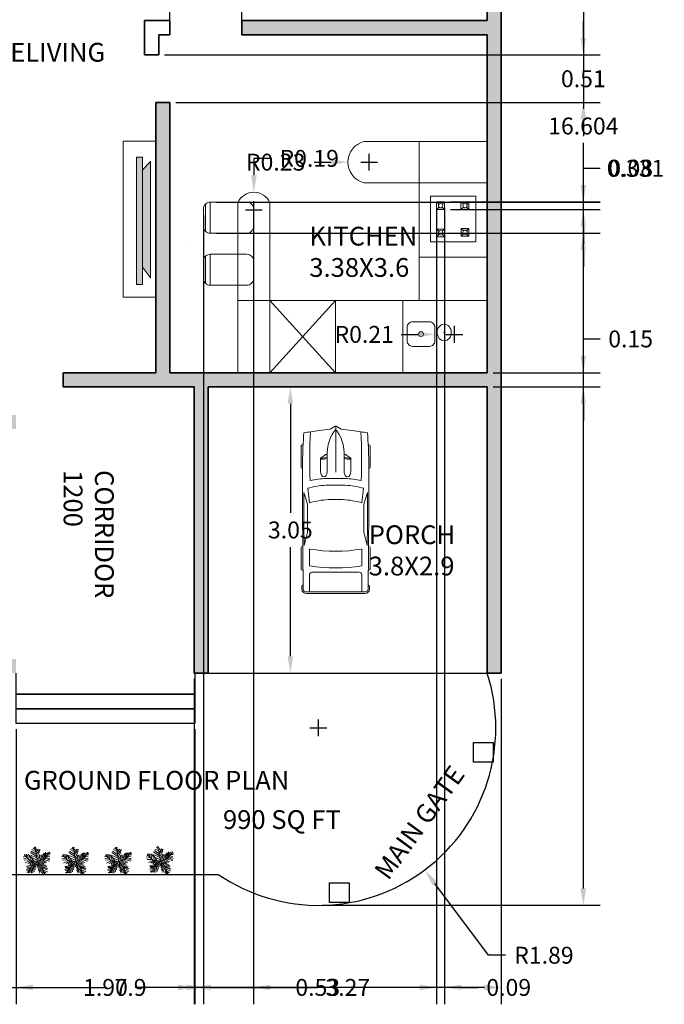
# Model space of a CAD drawing. Units: metres. Extents: x 36 to 56493, y 9 to 42849.
# Tile 2 of 5: x 56486.02 to 56492.89, y 42829.4 to 42839.88. Entities that reach past the tile are written whole.
import ezdxf

# ---------------------------------------------------------------- set-up
doc = ezdxf.new("R2010")
doc.units = ezdxf.units.M
doc.header["$MEASUREMENT"] = 0
for name, color, linetype, lineweight in [('A-ANNO-DIMS', 2, 'Continuous', 18), ('A-ANNO-TEXT', 7, 'Continuous', 25), ('A-AREA-IDEN', 7, 'Continuous', 18), ('A-EQPM', 8, 'Continuous', 18), ('A-EQPM-PATT', 8, 'Continuous', 13), ('A-FLOR', 7, 'Continuous', 25), ('A-FLOR-CASE', 9, 'Continuous', 18), ('A-FLOR-FIXT', 8, 'Continuous', 18), ('A-FLOR-STRS', 2, 'Continuous', 25), ('A-FURN', 8, 'Continuous', 18), ('A-WALL', 7, 'Continuous', 35), ('C-PKNG-VEHC', 9, 'Continuous', 13), ('C-PROP', 7, 'Continuous', 25), ('L-PLNT', 3, 'Continuous', 13)]:
    doc.layers.add(name, color=color, linetype=linetype, lineweight=lineweight)
doc.layers.add('A-WALL-PATT', color=30, linetype='Continuous', lineweight=13, true_color=0xf26722)
doc.styles.get("Standard").update_dxf_attribs({"font": 'arial.ttf'})
doc.dimstyles.get("Standard").update_dxf_attribs({"dimtxt": 0.18, "dimasz": 0.18, "dimexe": 0.18, "dimexo": 0.0625, "dimgap": 0.09, "dimtad": 0, "dimtih": 1, "dimtoh": 1, "dimdec": 0, "dimzin": 0, "dimdsep": 46, "dimtxsty": 'Standard', "dimcen": 0.09, "dimadec": 0, "dimazin": 0, "dimtfac": 1, "dimtdec": 0, "dimtofl": 0, "dimtmove": 0, "dimatfit": 3, "dimfxl": 1, "dimtolj": 1, "dimtzin": 0, "dimarcsym": 0})

# ---------------------------------------------------------------- blocks, each defined once
blk = doc.blocks.new('*U4')
for p, q in [((-5.114, 28.097), (-24.676, 40.636)), ((-7.288, 39.707), (-21.778, 46.673)), ((-8.737, 47.138), (-17.069, 52.711)), ((-10.186, 53.64), (-13.084, 55.962)), ((0, 0), (-10.5, 57)), ((-9.099, 51.782), (-6.563, 55.962)), ((-7.65, 43.423), (-2.578, 49.46)), ((-5.839, 35.992), (4.667, 48.067)), ((-5.114, 27.632), (10.463, 46.673)), ((-47.498, 19.737), (-55.83, 18.344)), ((-40.615, 13.7), (-55.105, 10.913)), ((-31.5, 4.5), (-52.5, 25.5)), ((-33.37, 6.269), (-52.207, 5.34)), ((-48.585, 21.131), (-49.309, 29.026)), ((-28.299, 3.483), (-47.86, -5.805)), ((-43.513, 28.561), (-42.427, 15.558)), ((-38.442, 26.239), (-34.819, 7.663)), ((-21.416, 3.018), (-38.079, -8.128)), ((-35.544, 28.097), (-24.314, 3.947)), ((0, 0), (-31.5, 4.5)), ((-14.533, 2.09), (-30.834, 25.31)), ((-15.982, 2.09), (-30.11, -9.521)), ((-3.665, 19.273), (-27.574, 35.527)), ((-24.314, 23.917), (-2.941, 13.7)), ((0, 0), (-22.5, -19.5)), ((-6.563, 1.161), (-21.416, -8.128)), ((-20.691, 13.7), (-1.129, 4.876)), ((-2.941, 16.486), (8.652, 37.85)), ((-1.129, 6.734), (9.014, 26.704)), ((0, 0), (27, 9)), ((0, 0), (18, -22.5)), ((3.942, 1.625), (11.187, 24.381)), ((6.478, 1.625), (26.04, -8.592)), ((10.101, 3.483), (17.708, 26.239)), ((11.187, 3.483), (30.749, -5.805)), ((16.259, 5.805), (23.142, 31.348)), ((18.07, 5.805), (35.096, -3.483)), ((22.055, 7.198), (27.489, 32.277)), ((24.229, 7.663), (46.688, 1.625)), ((27, 9), (48, 36)), ((27.127, 9.056), (31.112, 35.992)), ((29.662, 12.307), (48.137, 6.269)), ((31.836, 30.883), (32.561, 16.486)), ((33.285, 16.486), (48.862, 10.913)), ((35.096, 32.741), (37.27, 22.524)), ((36.183, 19.737), (48.137, 17.88)), ((38.719, 34.134), (41.979, 28.561)), ((40.53, 25.775), (48.862, 24.846)), ((43.791, 29.954), (51.036, 30.883)), ((44.153, 36.456), (45.239, 32.741)), ((-17.431, -15.094), (-42.789, -18.809)), ((-28.299, -29.026), (-42.789, -31.348)), ((-24.314, -21.596), (-42.427, -22.06)), ((-30.834, -34.135), (-42.427, -35.528)), ((-26.849, -26.24), (-40.253, -25.775)), ((-22.5, -19.5), (-37.5, -45)), ((-32.646, -36.921), (-31.921, -44.352)), ((-15.257, -12.772), (-30.11, -12.772)), ((-29.023, -30.884), (-27.936, -43.887)), ((-25.038, -23.918), (-22.865, -45.281)), ((-20.691, -18.345), (-17.793, -44.352)), ((-6.563, -5.805), (-19.967, -9.985)), ((-17.069, -15.094), (-12.721, -40.172)), ((-13.446, -11.378), (-8.737, -32.741)), ((-9.461, -8.592), (-6.201, -23.453)), ((-4.752, -3.483), (-3.665, -14.629)), ((2.493, -3.019), (-1.491, -20.202)), ((1.769, -2.555), (24.229, -9.521)), ((5.029, -6.27), (2.131, -25.775)), ((9.014, -11.378), (3.58, -35.992)), ((14.085, -16.951), (6.478, -40.172)), ((7.565, -9.056), (32.198, -14.629)), ((18.07, -22.524), (8.289, -45.745)), ((12.274, -15.094), (36.907, -18.809)), ((20.244, -30.419), (15.897, -44.816)), ((16.259, -19.738), (36.183, -22.989)), ((18, -22.5), (27, -52.5)), ((18.433, -22.524), (40.53, -29.026)), ((19.157, -25.311), (38.719, -33.206)), ((22.78, -37.85), (19.519, -48.532)), ((21.331, -32.741), (39.081, -40.636)), ((22.78, -38.314), (34.372, -44.816)), ((-34.457, -39.708), (-40.978, -42.494)), ((24.591, -45.745), (23.142, -50.854)), ((24.591, -43.423), (30.749, -47.603)), ((26.764, -49.925), (28.213, -50.854))]:
    blk.add_line(p, q)
blk = doc.blocks.new('*U6')
for p, q in [((21.1, 37.4), (21.1, 36.8)), ((46.6, 38.9), (22.4, 38.9)), ((47.8, 37.4), (47.8, 37.4)), ((88, 31.9), (74.8, 35.9)), ((134.3, 35.6), (119.3, 31.8)), ((135.5, 37.1), (135.5, 37.4)), ((136.7, 38.9), (160.9, 38.9)), ((162.1, 37.4), (162.1, 36.8)), ((186.5, -33.5), (186.5, 33.5)), ((70, 31.5), (86.4, 29.4)), ((138.4, 29.4), (157.2, 29.4)), ((164.5, 26.4), (164.5, -26.4)), ((186.5, 29.4), (167, 29.4)), ((188.4, -32.8), (188.4, 32.8)), ((32.1, 9.5), (32.1, 11.2)), ((32.3, 11.6), (36.1, 17.2)), ((36.1, 17.2), (50.9, 17.2)), ((3.3, 6.1), (0.1, 0.4)), ((29.8, 9.5), (51.7, 9.5)), ((58.9, -10.8), (58.9, 10.8)), ((66.6, -10.5), (66.6, 10.5)), ((82.7, 8.5), (82.7, -8.5)), ((186.5, -10.5), (186.5, 10.5)), ((0, 0), (51.7, 0)), ((0.1, -0.4), (3.3, -6.1)), ((29.8, -9.5), (51.7, -9.5)), ((32.1, -9.5), (32.1, -11.2)), ((32.3, -11.6), (36.1, -17.2)), ((36.1, -17.2), (50.9, -17.2)), ((86.4, -29.4), (70, -31.5)), ((88, -31.9), (74.8, -35.9)), ((134.3, -35.6), (119.3, -31.8)), ((157.2, -29.4), (138.4, -29.4)), ((167, -29.4), (186.5, -29.4)), ((21.1, -37.4), (21.1, -36.8)), ((46.6, -38.9), (22.4, -38.9)), ((47.8, -37.4), (47.8, -37.4)), ((135.5, -37.1), (135.5, -37.4)), ((136.7, -38.9), (160.9, -38.9)), ((162.1, -37.4), (162.1, -36.8))]:
    blk.add_line(p, q)
for centre, major_axis, ratio, start_param, end_param in [((266, -27.5), (0, 313.3), 0.842304, 1.367076, 1.39176), ((41.2, -490.9), (0, 528.2), 0.842304, 0.00281, 0.075598), ((22.4, 37.4), (0, -1.48), 0.842304, 3.141593, 4.712389), ((64.5, -10555.6), (0, 10593), 0.842304, -0.013397, 0.002797), ((46.6, 37.4), (0, 1.48), 0.842304, -1.570796, 0), ((64.5, -10555.6), (0, -10591.5), 0.842304, 3.133765, 3.140441), ((136.7, 37.4), (0, -1.48), 0.842304, 3.141593, 4.712389), ((160.9, 37.4), (0, 1.48), 0.842304, -1.570796, 0), ((180.6, 35.8), (0, 2.22), 0.842304, -0.013017, 1.249894), ((64.5, -10556.4), (0, 10595.3), 0.842304, -0.013397, -0.013017), ((184, 32.8), (0, -5.25), 0.842304, 1.570796, 3.128196), ((184, 33.5), (0, -2.96), 0.842304, 1.570796, 3.128196), ((259.2, -27.5), (0, -305.3), 0.842304, 4.528606, 4.561838), ((37.5, -594), (0, -623.3), 0.842304, 3.096046, 3.200911), ((134.4, 5.4), (0, -89.8), 0.842304, 4.449482, 4.652344), ((135.3, 5.4), (0, 81.8), 0.842304, 1.245306, 1.50788), ((149.6, 2.8), (0, -79.6), 0.842304, 4.372215, 4.640744), ((95.8, -3666.4), (0, -3698.2), 0.842304, 3.134049, 3.144098), ((17.1, 0), (0, 147), 0.842304, 4.511394, 4.913384), ((35.9, 0), (0, 147), 0.842304, 4.511394, 4.913384), ((167, 26.4), (0, 2.96), 0.842304, 0, 1.570796), ((-204.5, 52.4), (0, -251), 0.842304, 1.385369, 1.434372), ((32.7, 11.2), (0, 0.74), 0.842304, 0.879714, 1.570796), ((13, 17), (0, 27.4), 0.842304, 4.435146, 4.718221), ((14.2, 17), (0, 27.4), 0.842304, 4.435146, 4.718221), ((50.8, 13.3), (6.34, -0.36), 0.603834, -1.395552, 1.581315), ((0.6, 0), (0, -0.74), 0.842304, 4.131459, 5.293319), ((29.8, -46.7), (0, 56.2), 0.842304, 0, 0.590319), ((-204.5, -52.4), (0, 251), 0.842304, -1.434372, -1.385369), ((29.8, 46.7), (0, 56.2), 0.842304, 2.551274, 3.141593), ((13, -17), (0, -27.4), 0.842304, 1.564964, 1.848039), ((14.2, -17), (0, -27.4), 0.842304, 1.564964, 1.848039), ((134.4, -5.4), (0, -89.8), 0.842304, -1.510751, -1.307889), ((135.3, -5.4), (0, -81.8), 0.842304, -1.50788, -1.245306), ((149.6, -2.8), (0, -79.6), 0.842304, -1.499151, -1.230623), ((259.2, 27.5), (0, 305.3), 0.842304, 1.721348, 1.754579), ((32.7, -11.2), (0, -0.74), 0.842304, 4.712389, 5.403472), ((266, 27.5), (0, 313.3), 0.842304, 1.749832, 1.774517), ((37.5, 594), (0, -623.3), 0.842304, -0.059319, 0.045547), ((95.8, 3666.4), (0, -3698.2), 0.842304, -0.002505, 0.007544), ((167, -26.4), (0, -2.96), 0.842304, 4.712389, 6.283185), ((184, -32.8), (0, -5.25), 0.842304, 0.013397, 1.570796), ((41.2, 490.9), (0, -528.2), 0.842304, -0.075598, -0.00281), ((22.4, -37.4), (0, 1.48), 0.842304, 1.570796, 3.141593), ((64.5, 10555.6), (0, 10593), 0.842304, 3.138796, 3.15499), ((46.6, -37.4), (0, -1.48), 0.842304, 0, 1.570796), ((64.5, 10555.6), (0, -10591.5), 0.842304, 0.001152, 0.007828), ((136.7, -37.4), (0, -1.48), 0.842304, -1.570796, 0), ((160.9, -37.4), (0, 1.48), 0.842304, 3.141593, 4.712389), ((180.6, -35.8), (0, -2.22), 0.842304, -1.249894, 0.013017), ((64.5, 10556.4), (0, 10595.3), 0.842304, 3.15461, 3.15499), ((184, -33.5), (0, 2.96), 0.842304, 3.15499, 4.712389)]:
    blk.add_ellipse(centre, major_axis=major_axis, ratio=ratio, start_param=start_param, end_param=end_param)
at = {"extrusion": (0, 0, -1)}
blk.add_ellipse((50.8, -13.3), major_axis=(6.34, 0.36), ratio=0.603834, start_param=-1.395552, end_param=1.581315, dxfattribs=at)
blk = doc.blocks.new('HOB-BURNER')
for p, q in [((0, 0.081), (0.026, 0.057)), ((0, 0), (0.026, 0.025)), ((0.026, 0.025), (0.026, 0.025)), ((0.085, 0.081), (0.059, 0.057)), ((0.085, 0), (0.059, 0.025))]:
    blk.add_line(p, q)
blk.add_lwpolyline([(0, 0.081), (0, 0.081), (0.085, 0.081), (0.085, 0.081), (0.085, 0), (0.085, 0), (0, 0), (0, 0)], close=True)
blk.add_circle((0.043, 0.041), 0.0232)
blk = doc.blocks.new('COUNTER-STOOL')
for p, q in [((0.073, 0.331), (0.073, 0)), ((0.022, 0.31), (0.022, 0.022))]:
    blk.add_line(p, q)
blk.add_lwpolyline([(0, 0.258, -0.414214), (0.073, 0.331), (0.461, 0.331, -0.414214), (0.534, 0.258), (0.534, 0.073, -0.414214), (0.461, 0), (0.073, 0, -0.414214), (0, 0.073)], format="xyb", close=True)
blk = doc.blocks.new('*D16')
at = {"layer": 'A-ANNO-DIMS', "color": 0, "lineweight": -2, "transparency": 16777216}
for p, q in [((56491.156, 42832.861), (56491.156, 42829.395)), ((56483.256, 42830.716), (56483.256, 42829.395)), ((56483.436, 42829.575), (56486.953, 42829.575)), ((56490.976, 42829.575), (56487.46, 42829.575))]:
    blk.add_line(p, q, dxfattribs=at)
at = {"layer": 'A-ANNO-DIMS', "color": 0, "transparency": 16777216}
for points in [[(56483.436, 42829.605), (56483.436, 42829.545), (56483.256, 42829.575)], [(56490.976, 42829.605), (56490.976, 42829.545), (56491.156, 42829.575)]]:
    blk.add_solid(points, dxfattribs=at)
at = {"layer": 'Defpoints', "color": 0, "transparency": 16777216}
for p in [(56491.156, 42832.923), (56483.256, 42830.779), (56491.156, 42829.575)]:
    blk.add_point(p, dxfattribs=at)
at = {"layer": 'A-ANNO-DIMS', "color": 0, "transparency": 16777216, "insert": (56487.206, 42829.575), "char_height": 0.18, "attachment_point": 5}
blk.add_mtext('\\A1;7.9', dxfattribs=at)
blk = doc.blocks.new('*D17')
at = {"layer": 'A-ANNO-DIMS', "color": 0, "lineweight": -2, "transparency": 16777216}
for p, q in [((56491.219, 42847.053), (56492.211, 42847.053)), ((56492.031, 42846.873), (56492.031, 42838.933)), ((56492.031, 42830.63), (56492.031, 42838.57)), ((56489.311, 42830.45), (56492.211, 42830.45))]:
    blk.add_line(p, q, dxfattribs=at)
at = {"layer": 'A-ANNO-DIMS', "color": 0, "transparency": 16777216}
for points in [[(56492.001, 42846.873), (56492.061, 42846.873), (56492.031, 42847.053)], [(56492.001, 42830.63), (56492.061, 42830.63), (56492.031, 42830.45)]]:
    blk.add_solid(points, dxfattribs=at)
at = {"layer": 'Defpoints', "color": 0, "transparency": 16777216}
for p in [(56491.156, 42847.053), (56489.249, 42830.45), (56492.031, 42830.45)]:
    blk.add_point(p, dxfattribs=at)
at = {"layer": 'A-ANNO-DIMS', "color": 0, "transparency": 16777216, "insert": (56492.031, 42838.751), "char_height": 0.18, "attachment_point": 5}
blk.add_mtext('\\A1;16.604', dxfattribs=at)
blk = doc.blocks.new('*D20')
at = {"layer": 'A-ANNO-DIMS', "color": 0, "lineweight": -2, "transparency": 16777216}
for p, q in [((56485.987, 42832.325), (56485.987, 42829.395)), ((56487.891, 42832.325), (56487.891, 42829.395)), ((56486.167, 42829.575), (56486.624, 42829.575)), ((56487.711, 42829.575), (56487.254, 42829.575))]:
    blk.add_line(p, q, dxfattribs=at)
at = {"layer": 'A-ANNO-DIMS', "color": 0, "transparency": 16777216}
for points in [[(56486.167, 42829.605), (56486.167, 42829.545), (56485.987, 42829.575)], [(56487.711, 42829.605), (56487.711, 42829.545), (56487.891, 42829.575)]]:
    blk.add_solid(points, dxfattribs=at)
at = {"layer": 'Defpoints', "color": 0, "transparency": 16777216}
for p in [(56485.987, 42832.388), (56487.891, 42832.388), (56487.891, 42829.575)]:
    blk.add_point(p, dxfattribs=at)
at = {"layer": 'A-ANNO-DIMS', "color": 0, "transparency": 16777216, "insert": (56486.939, 42829.575), "char_height": 0.18, "attachment_point": 5}
blk.add_mtext('\\A1;1.90', dxfattribs=at)
blk = doc.blocks.new('*D21')
at = {"layer": 'A-ANNO-DIMS', "color": 0, "lineweight": -2, "transparency": 16777216}
for p, q in [((56487.885, 42832.861), (56487.885, 42829.395)), ((56491.156, 42832.861), (56491.156, 42829.395)), ((56488.065, 42829.575), (56489.197, 42829.575)), ((56490.976, 42829.575), (56489.844, 42829.575))]:
    blk.add_line(p, q, dxfattribs=at)
at = {"layer": 'A-ANNO-DIMS', "color": 0, "transparency": 16777216}
for points in [[(56488.065, 42829.605), (56488.065, 42829.545), (56487.885, 42829.575)], [(56490.976, 42829.605), (56490.976, 42829.545), (56491.156, 42829.575)]]:
    blk.add_solid(points, dxfattribs=at)
at = {"layer": 'Defpoints', "color": 0, "transparency": 16777216}
for p in [(56487.885, 42832.923), (56491.156, 42832.923), (56491.156, 42829.575)]:
    blk.add_point(p, dxfattribs=at)
at = {"layer": 'A-ANNO-DIMS', "color": 0, "transparency": 16777216, "insert": (56489.521, 42829.575), "char_height": 0.18, "attachment_point": 5}
blk.add_mtext('\\A1;3.27', dxfattribs=at)
blk = doc.blocks.new('*D22')
at = {"layer": 'A-ANNO-DIMS', "color": 0, "lineweight": -2, "transparency": 16777216}
for p, q in [((56488.097, 42835.973), (56489.089, 42835.973)), ((56488.909, 42835.793), (56488.909, 42834.63)), ((56488.909, 42833.103), (56488.909, 42834.266)), ((56488.097, 42832.923), (56489.089, 42832.923))]:
    blk.add_line(p, q, dxfattribs=at)
at = {"layer": 'A-ANNO-DIMS', "color": 0, "transparency": 16777216}
for points in [[(56488.879, 42835.793), (56488.939, 42835.793), (56488.909, 42835.973)], [(56488.879, 42833.103), (56488.939, 42833.103), (56488.909, 42832.923)]]:
    blk.add_solid(points, dxfattribs=at)
at = {"layer": 'Defpoints', "color": 0, "transparency": 16777216}
for p in [(56488.035, 42835.973), (56488.035, 42832.923), (56488.909, 42832.923)]:
    blk.add_point(p, dxfattribs=at)
at = {"layer": 'A-ANNO-DIMS', "color": 0, "transparency": 16777216, "insert": (56488.909, 42834.448), "char_height": 0.18, "attachment_point": 5}
blk.add_mtext('\\A1;3.05', dxfattribs=at)
blk = doc.blocks.new('*D37')
at = {"layer": 'A-ANNO-DIMS', "color": 0, "lineweight": -2, "transparency": 16777216}
for p, q in [((56487.983165, 42837.804951), (56487.983165, 42829.395107)), ((56488.516956, 42837.804951), (56488.516956, 42829.395107)), ((56487.803165, 42829.575107), (56487.623165, 42829.575107)), ((56488.696956, 42829.575107), (56488.876956, 42829.575107))]:
    blk.add_line(p, q, dxfattribs=at)
at = {"layer": 'A-ANNO-DIMS', "color": 0, "transparency": 16777216}
for points in [[(56487.803165, 42829.605107), (56487.803165, 42829.545107), (56487.983165, 42829.575107)], [(56488.696956, 42829.605107), (56488.696956, 42829.545107), (56488.516956, 42829.575107)]]:
    blk.add_solid(points, dxfattribs=at)
at = {"layer": 'Defpoints', "color": 0, "transparency": 16777216}
for p in [(56487.983165, 42837.867451), (56488.516956, 42837.867451), (56488.516956, 42829.575107)]:
    blk.add_point(p, dxfattribs=at)
at = {"layer": 'A-ANNO-DIMS', "color": 0, "transparency": 16777216, "insert": (56489.200735, 42829.575107), "char_height": 0.18, "attachment_point": 5}
blk.add_mtext('\\A1;0.53', dxfattribs=at)
blk = doc.blocks.new('*D38')
at = {"layer": 'A-ANNO-DIMS', "color": 0, "lineweight": -2, "transparency": 16777216}
for p, q in [((56492.031, 42838.12), (56492.031, 42838.3)), ((56492.031, 42838.3), (56492.211, 42838.3)), ((56488.119, 42837.94), (56492.211, 42837.94)), ((56488.119, 42837.609), (56492.211, 42837.609)), ((56492.031, 42837.429), (56492.031, 42837.249))]:
    blk.add_line(p, q, dxfattribs=at)
at = {"layer": 'A-ANNO-DIMS', "color": 0, "transparency": 16777216}
for points in [[(56492.001, 42838.12), (56492.061, 42838.12), (56492.031, 42837.94)], [(56492.001, 42837.429), (56492.061, 42837.429), (56492.031, 42837.609)]]:
    blk.add_solid(points, dxfattribs=at)
at = {"layer": 'Defpoints', "color": 0, "transparency": 16777216}
for p in [(56488.056, 42837.94), (56492.031, 42837.94), (56488.056, 42837.609)]:
    blk.add_point(p, dxfattribs=at)
at = {"layer": 'A-ANNO-DIMS', "color": 0, "transparency": 16777216, "insert": (56492.587, 42838.3), "char_height": 0.18, "attachment_point": 5}
blk.add_mtext('\\A1;0.331', dxfattribs=at)
blk = doc.blocks.new('*D39')
at = {"layer": 'A-ANNO-DIMS', "color": 0, "lineweight": -2, "transparency": 16777216}
for p, q in [((56490.467, 42837.88), (56490.467, 42829.395)), ((56490.552, 42837.88), (56490.552, 42829.395)), ((56490.287, 42829.575), (56490.107, 42829.575)), ((56490.732, 42829.575), (56490.912, 42829.575))]:
    blk.add_line(p, q, dxfattribs=at)
at = {"layer": 'A-ANNO-DIMS', "color": 0, "transparency": 16777216}
for points in [[(56490.287, 42829.605), (56490.287, 42829.545), (56490.467, 42829.575)], [(56490.732, 42829.605), (56490.732, 42829.545), (56490.552, 42829.575)]]:
    blk.add_solid(points, dxfattribs=at)
at = {"layer": 'Defpoints', "color": 0, "transparency": 16777216}
for p in [(56490.467, 42837.942), (56490.552, 42837.942), (56490.552, 42829.575)]:
    blk.add_point(p, dxfattribs=at)
at = {"layer": 'A-ANNO-DIMS', "color": 0, "transparency": 16777216, "insert": (56491.236, 42829.575), "char_height": 0.18, "attachment_point": 5}
blk.add_mtext('\\A1;0.09', dxfattribs=at)
blk = doc.blocks.new('*D40')
at = {"layer": 'A-ANNO-DIMS', "color": 0, "lineweight": -2, "transparency": 16777216}
for p, q in [((56492.031, 42838.122), (56492.031, 42838.302)), ((56492.031, 42838.302), (56492.211, 42838.302)), ((56490.615, 42837.942), (56492.211, 42837.942)), ((56490.615, 42837.861), (56492.211, 42837.861)), ((56492.031, 42837.681), (56492.031, 42837.501))]:
    blk.add_line(p, q, dxfattribs=at)
at = {"layer": 'A-ANNO-DIMS', "color": 0, "transparency": 16777216}
for points in [[(56492.001, 42838.122), (56492.061, 42838.122), (56492.031, 42837.942)], [(56492.001, 42837.681), (56492.061, 42837.681), (56492.031, 42837.861)]]:
    blk.add_solid(points, dxfattribs=at)
at = {"layer": 'Defpoints', "color": 0, "transparency": 16777216}
for p in [(56490.552, 42837.942), (56492.031, 42837.942), (56490.552, 42837.861)]:
    blk.add_point(p, dxfattribs=at)
at = {"layer": 'A-ANNO-DIMS', "color": 0, "transparency": 16777216, "insert": (56492.535, 42838.302), "char_height": 0.18, "attachment_point": 5}
blk.add_mtext('\\A1;0.08', dxfattribs=at)
blk = doc.blocks.new('*D67')
at = {"layer": 'A-ANNO-DIMS', "color": 0, "lineweight": -2, "transparency": 16777216}
for p, q in [((56487.626252, 42839.785791), (56487.626252, 42848.721953)), ((56488.392626, 42839.785791), (56488.392626, 42848.721953)), ((56487.446252, 42848.541953), (56487.266252, 42848.541953)), ((56488.572626, 42848.541953), (56488.752626, 42848.541953))]:
    blk.add_line(p, q, dxfattribs=at)
at = {"layer": 'A-ANNO-DIMS', "color": 0, "transparency": 16777216}
for points in [[(56487.446252, 42848.571953), (56487.446252, 42848.511953), (56487.626252, 42848.541953)], [(56488.572626, 42848.571953), (56488.572626, 42848.511953), (56488.392626, 42848.541953)]]:
    blk.add_solid(points, dxfattribs=at)
at = {"layer": 'Defpoints', "color": 0, "transparency": 16777216}
for p in [(56488.392626, 42848.541953), (56487.626252, 42839.723291), (56488.392626, 42839.723291)]:
    blk.add_point(p, dxfattribs=at)
at = {"layer": 'A-ANNO-DIMS', "color": 0, "transparency": 16777216, "insert": (56488.009439, 42848.541953), "char_height": 0.18, "attachment_point": 5}
blk.add_mtext('\\A1;0.77', dxfattribs=at)
blk = doc.blocks.new('*D68')
at = {"layer": 'A-ANNO-DIMS', "color": 0, "lineweight": -2, "transparency": 16777216}
for p, q in [((56492.031, 42839.688), (56492.031, 42839.868)), ((56487.569, 42839.508), (56492.211, 42839.508)), ((56487.689, 42839.001), (56492.211, 42839.001)), ((56492.031, 42838.821), (56492.031, 42838.641))]:
    blk.add_line(p, q, dxfattribs=at)
at = {"layer": 'A-ANNO-DIMS', "color": 0, "transparency": 16777216}
for points in [[(56492.001, 42839.688), (56492.061, 42839.688), (56492.031, 42839.508)], [(56492.001, 42838.821), (56492.061, 42838.821), (56492.031, 42839.001)]]:
    blk.add_solid(points, dxfattribs=at)
at = {"layer": 'Defpoints', "color": 0, "transparency": 16777216}
for p in [(56487.506, 42839.508), (56487.626, 42839.001), (56492.031, 42839.001)]:
    blk.add_point(p, dxfattribs=at)
at = {"layer": 'A-ANNO-DIMS', "color": 0, "transparency": 16777216, "insert": (56492.031, 42839.254), "char_height": 0.18, "attachment_point": 5}
blk.add_mtext('\\A1;0.51', dxfattribs=at)
blk = doc.blocks.new('*D69')
at = {"layer": 'A-ANNO-DIMS', "color": 0, "lineweight": -2, "transparency": 16777216}
for p, q in [((56492.031, 42836.303), (56492.031, 42836.483)), ((56492.031, 42836.483), (56492.211, 42836.483)), ((56491.069, 42836.123), (56492.211, 42836.123)), ((56491.069, 42835.973), (56492.211, 42835.973)), ((56492.031, 42835.793), (56492.031, 42835.613))]:
    blk.add_line(p, q, dxfattribs=at)
at = {"layer": 'A-ANNO-DIMS', "color": 0, "transparency": 16777216}
for points in [[(56492.001, 42836.303), (56492.061, 42836.303), (56492.031, 42836.123)], [(56492.001, 42835.793), (56492.061, 42835.793), (56492.031, 42835.973)]]:
    blk.add_solid(points, dxfattribs=at)
at = {"layer": 'Defpoints', "color": 0, "transparency": 16777216}
for p in [(56491.006, 42836.123), (56492.031, 42836.123), (56491.006, 42835.973)]:
    blk.add_point(p, dxfattribs=at)
at = {"layer": 'A-ANNO-DIMS', "color": 0, "transparency": 16777216, "insert": (56492.535, 42836.483), "char_height": 0.18, "attachment_point": 5}
blk.add_mtext('\\A1;0.15', dxfattribs=at)
blk = doc.blocks.new('*D70')
at = {"layer": 'A-ANNO-DIMS', "color": 0, "lineweight": -2, "transparency": 16777216}
for p, q in [((56489.208, 42832.25), (56489.208, 42832.43)), ((56489.118, 42832.34), (56489.298, 42832.34)), ((56491.021, 42829.918), (56490.449, 42830.682)), ((56491.201, 42829.918), (56491.021, 42829.918))]:
    blk.add_line(p, q, dxfattribs=at)
at = {"layer": 'A-ANNO-DIMS', "color": 0, "transparency": 16777216}
blk.add_solid([(56490.473, 42830.7), (56490.425, 42830.664), (56490.341, 42830.826)], dxfattribs=at)
at = {"layer": 'Defpoints', "color": 0, "transparency": 16777216}
for p in [(56489.208, 42832.34), (56490.341, 42830.826)]:
    blk.add_point(p, dxfattribs=at)
at = {"layer": 'A-ANNO-DIMS', "color": 0, "transparency": 16777216, "insert": (56491.611, 42829.918), "char_height": 0.18, "attachment_point": 5}
blk.add_mtext('\\A1;R1.89', dxfattribs=at)
blk = doc.blocks.new('*D72')
at = {"layer": 'A-ANNO-DIMS', "color": 0, "lineweight": -2, "transparency": 16777216}
for p, q in [((56489.162, 42838.366), (56489.342, 42838.366)), ((56489.659, 42838.366), (56489.839, 42838.366)), ((56489.749, 42838.276), (56489.749, 42838.456))]:
    blk.add_line(p, q, dxfattribs=at)
at = {"layer": 'A-ANNO-DIMS', "color": 0, "transparency": 16777216}
blk.add_solid([(56489.342, 42838.396), (56489.342, 42838.336), (56489.522, 42838.366)], dxfattribs=at)
at = {"layer": 'Defpoints', "color": 0, "transparency": 16777216}
for p in [(56489.522, 42838.366), (56489.749, 42838.366)]:
    blk.add_point(p, dxfattribs=at)
at = {"layer": 'A-ANNO-DIMS', "color": 0, "transparency": 16777216, "insert": (56488.752, 42838.366), "char_height": 0.18, "attachment_point": 5}
blk.add_mtext('\\A1;R0.23', dxfattribs=at)
blk = doc.blocks.new('*D73')
at = {"layer": 'A-ANNO-DIMS', "color": 0, "lineweight": -2, "transparency": 16777216}
for p, q in [((56490.657, 42836.441), (56490.657, 42836.621)), ((56490.089, 42836.531), (56490.269, 42836.531)), ((56490.567, 42836.531), (56490.747, 42836.531))]:
    blk.add_line(p, q, dxfattribs=at)
at = {"layer": 'A-ANNO-DIMS', "color": 0, "transparency": 16777216}
blk.add_solid([(56490.269, 42836.561), (56490.269, 42836.501), (56490.449, 42836.531)], dxfattribs=at)
at = {"layer": 'Defpoints', "color": 0, "transparency": 16777216}
for p in [(56490.449, 42836.531), (56490.657, 42836.531)]:
    blk.add_point(p, dxfattribs=at)
at = {"layer": 'A-ANNO-DIMS', "color": 0, "transparency": 16777216, "insert": (56489.696, 42836.531), "char_height": 0.18, "attachment_point": 5}
blk.add_mtext('\\A1;R0.21', dxfattribs=at)
blk = doc.blocks.new('*D74')
at = {"layer": 'A-ANNO-DIMS', "color": 0, "lineweight": -2, "transparency": 16777216}
for p, q in [((56488.7, 42838.406), (56488.52, 42838.406)), ((56488.52, 42838.406), (56488.52, 42838.226)), ((56488.52, 42837.769), (56488.52, 42837.949)), ((56488.43, 42837.859), (56488.61, 42837.859))]:
    blk.add_line(p, q, dxfattribs=at)
at = {"layer": 'A-ANNO-DIMS', "color": 0, "transparency": 16777216}
blk.add_solid([(56488.49, 42838.226), (56488.55, 42838.226), (56488.52, 42838.046)], dxfattribs=at)
at = {"layer": 'Defpoints', "color": 0, "transparency": 16777216}
for p in [(56488.52, 42838.046), (56488.52, 42837.859)]:
    blk.add_point(p, dxfattribs=at)
at = {"layer": 'A-ANNO-DIMS', "color": 0, "transparency": 16777216, "insert": (56489.11, 42838.406), "char_height": 0.18, "attachment_point": 5}
blk.add_mtext('\\A1;R0.19', dxfattribs=at)

msp = doc.modelspace()

# ---------------------------------------------------------------- hatches: boundary and pattern name
at = {"layer": 'A-EQPM-PATT'}
h = msp.add_hatch(color=256, dxfattribs=at)
h.dxf.hatch_style = 1
h.paths.add_polyline_path([(56487.4198, 42838.3725), (56487.3351, 42838.2832), (56487.3351, 42837.2475), (56487.4198, 42837.1338)])
h.paths.add_polyline_path([(56487.3351, 42838.4194), (56487.2693, 42838.4194), (56487.2693, 42837.0621), (56487.3351, 42837.0621)])
at = {"layer": 'A-WALL-PATT'}
h = msp.add_hatch(color=256, dxfattribs=at)
h.dxf.hatch_style = 1
edge = h.paths.add_edge_path()
edge.add_line((56483.5429, 42845.6533), (56483.4063, 42845.6533))
edge.add_line((56483.4063, 42845.6533), (56483.4063, 42846.9033))
edge.add_line((56483.4063, 42846.9033), (56483.63, 42846.9033))
edge.add_ellipse((56483.6664, 42846.7323), major_axis=(0.2141, -0.003), ratio=0.809245, start_angle=94.07135, end_angle=102.818, ccw=False)
edge.add_line((56483.6565, 42846.9062), (56483.6565, 42846.9056))
edge.add_line((56483.6565, 42846.9056), (56483.6615, 42846.9056))
edge.add_ellipse((56483.6664, 42846.7323), major_axis=(0.2141, -0.003), ratio=0.809245, start_angle=90, end_angle=92.42655, ccw=False)
edge.add_line((56483.6812, 42846.9058), (56483.6812, 42846.9052))
edge.add_ellipse((56483.6664, 42846.7323), major_axis=(0.2141, -0.003), ratio=0.809245, start_angle=79.57494, end_angle=85.92601, ccw=False)
edge.add_line((56483.7048, 42846.9033), (56484.1418, 42846.9033))
edge.add_line((56484.1418, 42846.9033), (56484.1418, 42847.0533))
edge.add_line((56484.1418, 42847.0533), (56483.2563, 42847.0533))
edge.add_line((56483.2563, 42847.0533), (56483.2563, 42844.1391))
edge.add_line((56483.2563, 42844.1391), (56483.4063, 42844.1391))
edge.add_line((56483.4063, 42844.1391), (56483.4063, 42844.2368))
edge.add_line((56483.4063, 42844.2368), (56483.4063, 42845.5033))
edge.add_line((56483.4063, 42845.5033), (56483.5429, 42845.5033))
edge.add_line((56483.5429, 42845.5033), (56483.5429, 42845.6533))
edge = h.paths.add_edge_path(flags=0)
edge.add_line((56488.6347, 42847.0533), (56486.6826, 42847.0533))
edge.add_line((56486.6826, 42847.0533), (56486.6826, 42846.9033))
edge.add_line((56486.6826, 42846.9033), (56486.9892, 42846.9033))
edge.add_ellipse((56487.0257, 42846.7323), major_axis=(0.2141, -0.003), ratio=0.809245, start_angle=94.07135, end_angle=102.818, ccw=False)
edge.add_line((56487.0157, 42846.9062), (56487.0157, 42846.9056))
edge.add_line((56487.0157, 42846.9056), (56487.0207, 42846.9056))
edge.add_ellipse((56487.0257, 42846.7323), major_axis=(0.2141, -0.003), ratio=0.809245, start_angle=90, end_angle=92.42655, ccw=False)
edge.add_line((56487.0404, 42846.9058), (56487.0404, 42846.9052))
edge.add_ellipse((56487.0257, 42846.7323), major_axis=(0.2141, -0.003), ratio=0.809245, start_angle=79.57494, end_angle=85.92601, ccw=False)
edge.add_line((56487.064, 42846.9033), (56487.3563, 42846.9033))
edge.add_line((56487.3563, 42846.9033), (56487.3563, 42846.6728))
edge.add_line((56487.3563, 42846.6728), (56487.5063, 42846.6728))
edge.add_line((56487.5063, 42846.6728), (56487.5063, 42846.9033))
edge.add_line((56487.5063, 42846.9033), (56488.6347, 42846.9033))
edge.add_line((56488.6347, 42846.9033), (56488.6347, 42847.0533))
h.paths.add_polyline_path([(56486.2245, 42847.0533), (56484.665, 42847.0533), (56484.665, 42846.9033), (56485.4063, 42846.9033), (56485.4063, 42845.6533), (56484.2087, 42845.6533), (56484.2087, 42845.5033), (56487.3563, 42845.5033), (56487.3563, 42844.954), (56487.3563, 42843.021), (56487.5063, 42843.021), (56487.5063, 42843.2533), (56489.9401, 42843.2533), (56489.9401, 42843.4033), (56487.5063, 42843.4033), (56487.5063, 42845.6238), (56487.5063, 42845.6533), (56487.5063, 42845.9366), (56487.3563, 42845.9366), (56487.3563, 42845.6533), (56485.5563, 42845.6533), (56485.5563, 42846.9033), (56486.2245, 42846.9033)])
h.paths.add_polyline_path([(56491.1563, 42847.0533), (56489.9198, 42847.0533), (56489.9198, 42846.9033), (56489.9717, 42846.9033), (56491.0063, 42846.9033), (56491.0063, 42845.887), (56491.1563, 42845.887)])
h.paths.add_polyline_path([(56491.1563, 42844.3264), (56491.0063, 42844.3264), (56491.0063, 42843.4033), (56490.7805, 42843.4033), (56490.7805, 42843.2533), (56491.0063, 42843.2533), (56491.0063, 42839.8733), (56488.3926, 42839.8733), (56488.3926, 42839.7233), (56491.0063, 42839.7233), (56491.0063, 42836.1233), (56487.6263, 42836.1233), (56487.6263, 42839.0009), (56487.4763, 42839.0009), (56487.4763, 42836.1233), (56486.4863, 42836.1233), (56486.4863, 42835.9733), (56487.4763, 42835.9733), (56487.8849, 42835.9733), (56487.8849, 42832.9233), (56487.8913, 42832.9233), (56488.0349, 42832.9233), (56488.0349, 42833.0733), (56488.0349, 42835.9733), (56491.0063, 42835.9733), (56491.0063, 42833.0733), (56491.0063, 42832.9233), (56491.1563, 42832.9233), (56491.1563, 42835.9733)])
h.paths.add_polyline_path([(56483.4063, 42842.8378), (56483.2563, 42842.8378), (56483.2563, 42841.5433), (56483.2563, 42840.8898), (56483.4063, 42840.8898), (56483.4063, 42841.3933), (56485.0063, 42841.3933), (56485.0063, 42841.2426), (56485.1563, 42841.2426), (56485.1563, 42841.3933), (56487.3563, 42841.3933), (56487.5063, 42841.3933), (56487.5063, 42841.9264), (56487.3563, 42841.9264), (56487.3563, 42841.5433), (56483.4063, 42841.5433)])
h.paths.add_polyline_path([(56485.1563, 42840.351), (56485.0063, 42840.351), (56485.0063, 42839.8933), (56483.4063, 42839.8933), (56483.4063, 42840.3779), (56483.2563, 42840.3779), (56483.2563, 42839.8933), (56483.2563, 42838.6997), (56483.4063, 42838.6997), (56483.4063, 42839.7433), (56485.1563, 42839.7433)])
h.paths.add_polyline_path([(56483.4063, 42836.7612), (56483.2563, 42836.7612), (56483.2563, 42835.6733), (56483.2563, 42834.2533), (56483.2563, 42832.9233), (56485.9871, 42832.9233), (56485.9871, 42833.0733), (56483.4063, 42833.0733), (56483.4063, 42834.2533), (56483.4063, 42835.5233), (56485.4763, 42835.5233), (56485.9871, 42835.5233), (56485.9871, 42835.6733), (56485.6263, 42835.6733), (56483.4063, 42835.6733)])

# ---------------------------------------------------------------- linework, layer by layer
at = {"layer": 'A-EQPM'}
for p, q in [((56487.3351, 42838.2832), (56487.4198, 42838.3725)), ((56487.4198, 42838.3725), (56487.4198, 42837.1338)), ((56487.4198, 42837.1338), (56487.3351, 42837.2475))]:
    msp.add_line(p, q, dxfattribs=at)
for points in [[(56487.4763, 42838.5892), (56487.4763, 42838.5892), (56487.127, 42838.5892), (56487.127, 42838.5892), (56487.127, 42836.9285), (56487.127, 42836.9285), (56487.4763, 42836.9285), (56487.4763, 42836.9285)], [(56487.3351, 42838.4194), (56487.3351, 42838.4194), (56487.2693, 42838.4194), (56487.2693, 42838.4194), (56487.2693, 42837.0621), (56487.2693, 42837.0621), (56487.3351, 42837.0621), (56487.3351, 42837.0621)], [(56490.4027, 42838.0049), (56490.4027, 42838.0049), (56490.8862, 42838.0049), (56490.8862, 42838.0049), (56490.8862, 42837.5166), (56490.8862, 42837.5166), (56490.4027, 42837.5166), (56490.4027, 42837.5166)]]:
    msp.add_lwpolyline(points, close=True, dxfattribs=at)
at = {"layer": 'A-FLOR'}
msp.add_line((56488.0349, 42832.9233), (56491.0063, 42832.9233), dxfattribs=at)
at = {"layer": 'A-FLOR-CASE'}
for p, q in [((56490.282, 42838.1467), (56490.282, 42838.5858)), ((56488.35, 42836.8923), (56488.35, 42837.9361)), ((56488.6898, 42837.9361), (56488.6898, 42836.8923)), ((56490.282, 42837.3521), (56491.0063, 42837.3521)), ((56491.0063, 42836.8923), (56488.35, 42836.8923)), ((56488.35, 42836.8923), (56488.35, 42836.1233)), ((56488.6898, 42836.8923), (56489.3886, 42836.1233)), ((56489.3886, 42836.8923), (56488.6898, 42836.1233))]:
    msp.add_line(p, q, dxfattribs=at)
msp.add_lwpolyline([(56489.6919, 42838.5858), (56489.6919, 42838.5858), (56491.0063, 42838.5858), (56491.0063, 42838.5858), (56491.0063, 42838.1467), (56491.0063, 42838.1467), (56489.6919, 42838.1467), (56489.6919, 42838.1467)], dxfattribs=at)
for points in [[(56491.0063, 42836.8923), (56491.0063, 42836.8923), (56490.282, 42836.8923), (56490.282, 42836.8923), (56490.282, 42838.1467), (56490.282, 42838.1467), (56491.0063, 42838.1467), (56491.0063, 42838.1467)], [(56487.7949, 42837.5288), (56487.7949, 42837.5288)], [(56488.35, 42836.8923), (56488.6898, 42836.8923), (56488.6898, 42836.1233), (56488.35, 42836.1233)], [(56488.6898, 42836.8923), (56489.3886, 42836.8923), (56489.3886, 42836.1233), (56488.6898, 42836.1233)], [(56489.3886, 42836.8923), (56490.1066, 42836.8923), (56490.1066, 42836.1233), (56489.3886, 42836.1233)]]:
    msp.add_lwpolyline(points, close=True, dxfattribs=at)
for centre, radius, start, end in [((56489.749, 42838.3663), 0.2269, 104.60072, 255.39928), ((56488.5199, 42837.8593), 0.1864, 24.3046, 155.6954)]:
    msp.add_arc(centre, radius, start, end, dxfattribs=at)
at = {"layer": 'A-FLOR-FIXT'}
msp.add_lwpolyline([(56490.1536, 42836.6075, -0.4142136), (56490.2113, 42836.6651), (56490.3909, 42836.6651, -0.4142136), (56490.4486, 42836.6075), (56490.4486, 42836.4612, -0.4142136), (56490.3909, 42836.4036), (56490.2113, 42836.4036, -0.4142136), (56490.1536, 42836.4612)], format="xyb", close=True, dxfattribs=at)
for centre, radius in [((56490.3011, 42836.5343), 0.0259), ((56490.5483, 42836.5513), 0.00495)]:
    msp.add_circle(centre, radius, dxfattribs=at)
msp.add_arc((56490.6571, 42836.531), 0.2085, 179.18506, 180.81494, dxfattribs=at)
msp.add_ellipse((56490.5483, 42836.5513), major_axis=(0.0017, -0.0883), ratio=0.8566459, dxfattribs=at)
at = {"layer": 'A-FLOR-STRS'}
msp.add_lwpolyline([(56487.8849, 42832.9233), (56487.8913, 42832.9233), (56487.8913, 42832.9233), (56487.8913, 42832.6987), (56487.8913, 42832.6987), (56485.9871, 42832.6987), (56485.9871, 42832.6987), (56485.9871, 42832.9233)], dxfattribs=at)
for points in [[(56485.9871, 42832.6987), (56485.9871, 42832.6987), (56487.8914, 42832.6987), (56487.8914, 42832.6987), (56487.8914, 42832.5432), (56487.8914, 42832.5432), (56485.9871, 42832.5432), (56485.9871, 42832.5432)], [(56485.9871, 42832.5432), (56485.9871, 42832.5432), (56487.8914, 42832.5432), (56487.8914, 42832.5432), (56487.8914, 42832.3877), (56487.8914, 42832.3877), (56485.9871, 42832.3877), (56485.9871, 42832.3877)]]:
    msp.add_lwpolyline(points, close=True, dxfattribs=at)
at = {"layer": 'A-WALL'}
for p, q in [((56491.1563, 42847.0533), (56491.1563, 42832.9233)), ((56491.0063, 42843.2533), (56491.0063, 42839.8733)), ((56487.3563, 42839.8733), (56487.3563, 42839.508)), ((56487.5063, 42839.8733), (56487.3563, 42839.8733)), ((56487.6263, 42839.8733), (56487.5063, 42839.8733)), ((56487.6263, 42839.7233), (56487.6263, 42839.8733)), ((56491.0063, 42839.8733), (56488.3926, 42839.8733)), ((56488.3926, 42839.8733), (56488.3926, 42839.7233)), ((56487.6263, 42839.7233), (56487.5063, 42839.7233)), ((56487.5063, 42839.7233), (56487.5063, 42839.508)), ((56491.0063, 42839.7233), (56488.3926, 42839.7233)), ((56491.0063, 42839.7233), (56491.0063, 42836.1233)), ((56491.1563, 42839.7233), (56491.1563, 42836.1233)), ((56487.3563, 42839.508), (56487.5063, 42839.508)), ((56487.4763, 42836.1233), (56487.4763, 42839.0009)), ((56487.4763, 42839.0009), (56487.6263, 42839.0009)), ((56487.6263, 42836.1233), (56487.6263, 42839.0009)), ((56487.4763, 42836.1233), (56486.4863, 42836.1233)), ((56486.4863, 42835.9733), (56486.4863, 42836.1233)), ((56491.0063, 42836.1233), (56487.6263, 42836.1233)), ((56487.4763, 42835.9733), (56486.4863, 42835.9733)), ((56487.8849, 42835.9733), (56487.4763, 42835.9733)), ((56487.8849, 42832.9233), (56487.8849, 42835.9733)), ((56491.0063, 42835.9733), (56488.0349, 42835.9733)), ((56488.0349, 42833.0733), (56488.0349, 42835.9733)), ((56491.0063, 42835.9733), (56491.0063, 42833.0733)), ((56491.1563, 42835.9733), (56491.1563, 42832.9233)), ((56488.0349, 42833.0733), (56488.0349, 42832.9233)), ((56491.0063, 42833.0733), (56491.0063, 42832.9233)), ((56488.0349, 42832.9233), (56487.8849, 42832.9233)), ((56491.1563, 42832.9233), (56491.0063, 42832.9233))]:
    msp.add_line(p, q, dxfattribs=at)
at = {"layer": 'C-PROP'}
msp.add_line((56483.2563, 42830.7787), (56488.1411, 42830.7787), dxfattribs=at)
for points in [[(56491.0714, 42831.9753), (56491.0714, 42831.9753), (56490.862, 42831.9753), (56490.862, 42831.9753), (56490.862, 42832.1856), (56490.862, 42832.1856), (56491.0714, 42832.1856), (56491.0714, 42832.1856)], [(56489.5366, 42830.478), (56489.5366, 42830.478), (56489.3272, 42830.478), (56489.3272, 42830.478), (56489.3272, 42830.6882), (56489.3272, 42830.6882), (56489.5366, 42830.6882), (56489.5366, 42830.6882)]]:
    msp.add_lwpolyline(points, close=True, dxfattribs=at)
msp.add_arc((56489.2077, 42832.3399), 1.8908, 235.66035, 17.97049, dxfattribs=at)

# ---------------------------------------------------------------- block references
at = {"layer": 'A-EQPM'}
for p in [(56490.467, 42837.861), (56490.7273, 42837.861), (56490.467, 42837.572), (56490.7275, 42837.5781)]:
    msp.add_blockref('HOB-BURNER', p, dxfattribs=at)
at = {"layer": 'A-FURN'}
for p in [(56487.983, 42837.609), (56487.983, 42837.0538)]:
    msp.add_blockref('COUNTER-STOOL', p, dxfattribs=at)
at = {"layer": 'C-PKNG-VEHC', "xscale": 0.009454409230489, "yscale": 0.009454409230489, "zscale": 0.009454409230489, "rotation": 270}
msp.add_blockref('*U6', (56489.3918, 42835.5536), dxfattribs=at)
at = {"layer": 'L-PLNT', "xscale": 0.0027152007263879, "yscale": 0.0027152007263879, "zscale": 0.0027152007263879}
for p in [(56486.2139, 42830.9167), (56486.6228, 42830.9158), (56487.0806, 42830.9158), (56487.5266, 42830.9219)]:
    msp.add_blockref('*U4', p, dxfattribs=at)

# ---------------------------------------------------------------- texts
at = {"layer": 'A-ANNO-TEXT', "insert": (56486.0694, 42831.8816), "char_height": 0.2, "attachment_point": 1}
msp.add_mtext_dynamic_manual_height_columns('GROUND FLOOR PLAN', width=4.913662, gutter_width=1, heights=[0], dxfattribs=at)
at = {"layer": 'A-ANNO-TEXT', "insert": (56489.7906, 42830.8229), "char_height": 0.2, "attachment_point": 1, "rotation": 54.00752}
msp.add_mtext_dynamic_manual_height_columns('MAIN GATE', width=1.85462, gutter_width=1, heights=[0], dxfattribs=at)
at = {"layer": 'A-AREA-IDEN', "char_height": 0.2, "attachment_point": 1}
for s, width, insert in [('JUMBO SIZELIVING\\P5.25X4.07', 2.576018, (56484.5098, 42839.6363)), ('KITCHEN\\P3.38X3.6', 0.817901, (56489.111, 42837.6774)), ('PORCH\\P3.8X2.9', 0.817901, (56489.7441, 42834.4969)), ('990 SQ FT', 1.389776, (56488.1908, 42831.463))]:
    msp.add_mtext_dynamic_manual_height_columns(s, width=width, gutter_width=1, heights=[0], dxfattribs=dict(at, insert=insert))
at = {"layer": 'A-AREA-IDEN', "insert": (56487.027, 42835.086), "char_height": 0.2, "attachment_point": 1, "rotation": 270}
msp.add_mtext_dynamic_manual_height_columns('CORRIDOR\\P1200', width=0.817901, gutter_width=1, heights=[0], dxfattribs=at)

# ---------------------------------------------------------------- dimensions: what is measured, and where the dimension line sits
at = {"layer": 'A-ANNO-DIMS'}
for base, p1, p2, override, picture, middle in [((56488.3926, 42848.542), (56487.6263, 42839.7233), (56488.3926, 42839.7233), {"dimdec": 2, "dimlfac": 1, "dimrnd": 0, "dimzin": 0, "dimdsep": 46, "dimlunit": 2}, '*D67', (56488.0094, 42848.542)), ((56490.5524, 42829.5751), (56490.4667, 42837.9423), (56490.5524, 42837.9423), {"dimdec": 2, "dimlfac": 1, "dimrnd": 0, "dimzin": 0, "dimdsep": 46, "dimlunit": 2}, '*D39', (56491.2363, 42829.5751)), ((56488.517, 42829.5751), (56487.9832, 42837.8675), (56488.517, 42837.8675), {"dimdec": 2, "dimlfac": 1, "dimrnd": 0, "dimzin": 0, "dimdsep": 46, "dimlunit": 2}, '*D37', (56489.2007, 42829.5751)), ((56491.1563, 42829.5751), (56483.2563, 42830.7787), (56491.1563, 42832.9233), {"dimdec": 1, "dimlfac": 1, "dimrnd": 0, "dimzin": 0, "dimdsep": 46, "dimlunit": 2}, '*D16', (56487.2063, 42829.5751)), ((56491.1563, 42829.5751), (56487.8849, 42832.9233), (56491.1563, 42832.9233), {"dimdec": 2, "dimlfac": 1, "dimrnd": 0, "dimzin": 0, "dimdsep": 46, "dimlunit": 2}, '*D21', (56489.5206, 42829.5751)), ((56487.8914, 42829.5751), (56485.9871, 42832.3877), (56487.8914, 42832.3877), {"dimdec": 2, "dimlfac": 1, "dimrnd": 0, "dimzin": 0, "dimdsep": 46, "dimlunit": 2}, '*D20', (56486.9392, 42829.5751))]:
    dim = msp.add_linear_dim(base=base, p1=p1, p2=p2, dimstyle='Standard', override=override, dxfattribs=at)
    dim.commit()
    dim.dimension.update_dxf_attribs({"geometry": picture, "text_midpoint": middle})
for base, p1, p2, angle, override, picture, middle in [((56492.0308, 42830.4496), (56491.1563, 42847.0533), (56489.2486, 42830.4496), 90, {"dimdec": 3, "dimlfac": 1, "dimrnd": 0, "dimzin": 0, "dimdsep": 46, "dimlunit": 2}, '*D17', (56492.0308, 42838.7514)), ((56492.0308, 42839.0009), (56487.5063, 42839.508), (56487.6263, 42839.0009), 90, {"dimdec": 2, "dimlfac": 1, "dimrnd": 0, "dimzin": 0, "dimdsep": 46, "dimlunit": 2}, '*D68', (56492.0308, 42839.2544)), ((56492.0308, 42837.9404), (56488.0561, 42837.6094), (56488.0561, 42837.9404), 90, {"dimdec": 3, "dimlfac": 1, "dimrnd": 0, "dimzin": 0, "dimdsep": 46, "dimlunit": 2}, '*D38', (56492.5871, 42838.3004)), ((56492.0308, 42837.9423), (56490.5524, 42837.8609), (56490.5524, 42837.9423), 90, {"dimdec": 2, "dimlfac": 1, "dimrnd": 0, "dimzin": 0, "dimdsep": 46, "dimlunit": 2}, '*D40', (56492.5347, 42838.3023)), ((56492.0308, 42836.1233), (56491.0063, 42835.9733), (56491.0063, 42836.1233), 90, {"dimdec": 2, "dimlfac": 1, "dimrnd": 0, "dimzin": 0, "dimdsep": 46, "dimlunit": 2}, '*D69', (56492.5352, 42836.4833)), ((56488.9094, 42832.9233), (56488.0349, 42835.9733), (56488.0349, 42832.9233), 270, {"dimdec": 2, "dimlfac": 1, "dimrnd": 0, "dimzin": 0, "dimdsep": 46, "dimlunit": 2}, '*D22', (56488.9094, 42834.4483))]:
    dim = msp.add_linear_dim(base=base, p1=p1, p2=p2, angle=angle, dimstyle='Standard', override=override, dxfattribs=at)
    dim.commit()
    dim.dimension.update_dxf_attribs({"geometry": picture, "text_midpoint": middle})
for center, mpoint, picture, middle in [((56488.5199, 42837.8593), (56488.52, 42838.0458), '*D74', (56489.1102, 42838.4058)), ((56489.749, 42838.3663), (56489.5222, 42838.366), '*D72', (56488.7523, 42838.3656)), ((56490.6571, 42836.531), (56490.4486, 42836.531), '*D73', (56489.696, 42836.5309))]:
    dim = msp.add_radius_dim(center=center, mpoint=mpoint, dimstyle='Standard', override={"dimdec": 2, "dimlfac": 1, "dimrnd": 0, "dimzin": 0, "dimdsep": 46, "dimlunit": 2}, dxfattribs=at)
    dim.commit()
    dim.dimension.update_dxf_attribs({"geometry": picture, "text_midpoint": middle})
dim = msp.add_radius_dim(center=(56489.2077, 42832.3399), mpoint=(56490.3408, 42830.8263), dimstyle='Standard', override={"dimdec": 2, "dimlfac": 1, "dimrnd": 0, "dimzin": 0, "dimdsep": 46, "dimlunit": 2}, dxfattribs=at)
dim.commit()
dim.dimension.update_dxf_attribs({"geometry": '*D70', "text_midpoint": (56491.6107, 42829.9181), "dimtype": 164})

doc.saveas('drawing.dxf')
